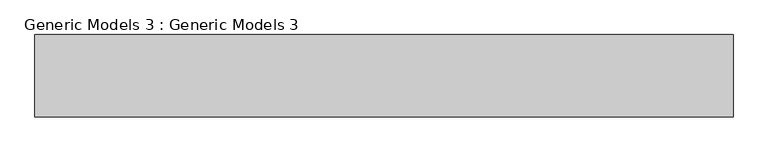
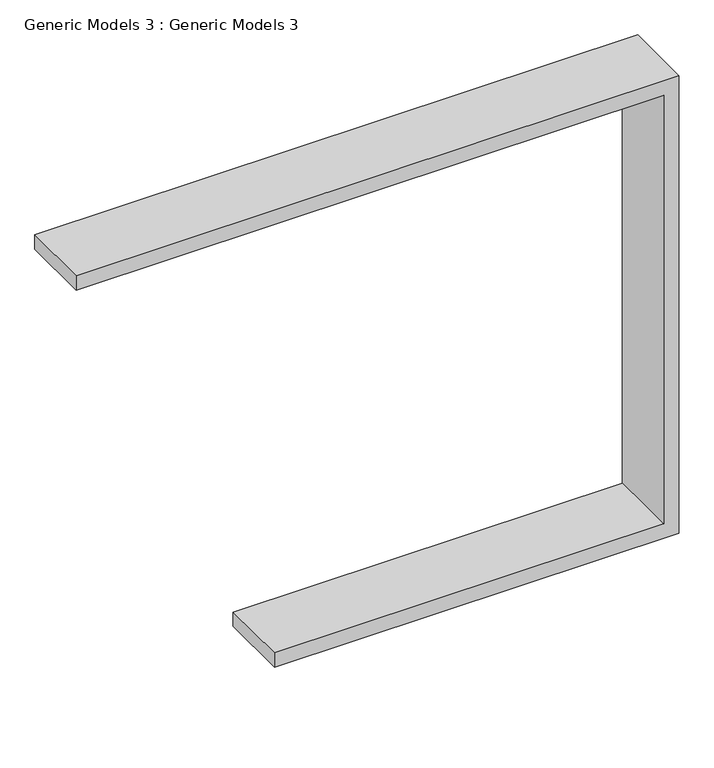
"""IFC4 building model written with IfcOpenShell, lengths in millimetres: proxy geometry, Generic Models 3 : Generic Models 3."""

from ifc_helpers import new_model, si_unit, frame, origin, place, context, project, spatial, polyline, outline, extrude, source, transform, mapped, element, save


def generic_models_3_generic_models_3_22da3405(model_context):
    return source(origin(), model_context, "Body", "SweptSolid", [
        extrude(outline(polyline([(4419.6, 8948.2271331), (4419.6, 3118.9271331), (4191.0, 3118.9271331), (4191.0, 9176.8271331), (4419.6, 9176.8271331), (11430.0, 9176.8271331), (11430.0, 147.1271331), (11201.4, 147.1271331), (11201.4, 8948.2271331), (4419.6, 8948.2271331)])), frame((0.0, -13042.5643494, 0.0), z_axis=(0.0, 1.0, 0.0), x_axis=(0.0, 0.0, 1.0)), (0.0, 0.0, 1.0), 1066.8),
    ])


if __name__ == "__main__":
    model = new_model("IFC4")
    model_context = context("Model", 3, world=origin())
    ifc_project = project(units=[si_unit("LENGTHUNIT", "METRE", prefix="MILLI")], contexts=[model_context])
    site = spatial("IfcSite", under=ifc_project)
    building = spatial("IfcBuilding", under=site)
    placement = place(None, origin())
    generic_models_3_generic_models_3_shape = generic_models_3_generic_models_3_22da3405(model_context)
    element("IfcBuildingElementProxy", 1, Name="Generic Models 3 : Generic Models 3", ObjectType="Generic Models 3 : Generic Models 3", at=placement, inside=building, context=model_context, shape_type="MappedRepresentation", body=[
        mapped(generic_models_3_generic_models_3_shape, transform((0.0, 0.0, 0.0), x_axis=(1.0, 0.0, 0.0), y_axis=(0.0, 1.0, 0.0), z_axis=(0.0, 0.0, 1.0))),
    ])
    save(model, "model.ifc")
